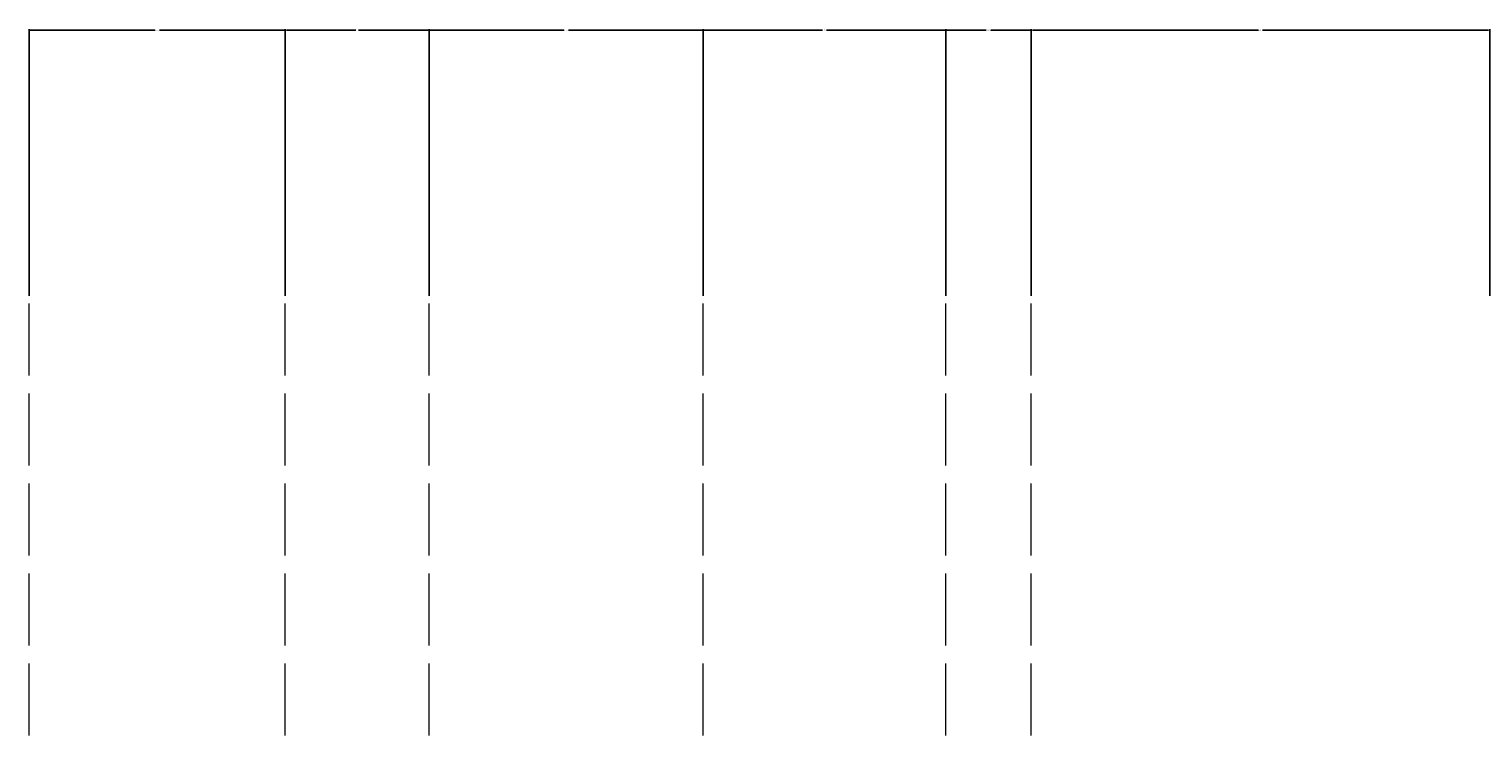
# Model space of a CAD drawing. Units: inches. Extents: x 1159 to 4240, y 1112 to 2085.
# Tile 7 of 13: x 1293 to 1535, y 1968 to 2085. Entities that reach past the tile are written whole.
import ezdxf

# ---------------------------------------------------------------- set-up
doc = ezdxf.new("R2010")
doc.units = ezdxf.units.IN
doc.linetypes.add('ACAD_ISO02W100', pattern=[15, 12, -3])
doc.layers.add('A-ANNO-DIMS', color=2, linetype='Continuous', lineweight=18)
doc.layers.add('A-GRID', color=8, linetype='ACAD_ISO02W100', lineweight=13)
doc.styles.get("Standard").update_dxf_attribs({"font": 'arial.ttf'})
doc.dimstyles.get("Standard").update_dxf_attribs({"dimtxt": 0.18, "dimasz": 0.18, "dimexe": 0.18, "dimexo": 0.0625, "dimgap": 0.09, "dimtad": 0, "dimtih": 1, "dimtoh": 1, "dimdec": 4, "dimzin": 0, "dimdsep": 46, "dimtxsty": 'Standard', "dimcen": 0.09, "dimadec": 0, "dimazin": 0, "dimtfac": 1, "dimtdec": 4, "dimtofl": 0, "dimtmove": 0, "dimatfit": 3, "dimfxl": 1, "dimtolj": 1, "dimtzin": 0, "dimarcsym": 0})

# ---------------------------------------------------------------- blocks, each defined once
blk = doc.blocks.new('HOUSE-35x60-SETTING-OUT-GRID')
for p, q in [((89.32, 0), (89.32, 883.25)), ((132.07, 0), (132.07, 883.25)), ((156.07, 0), (156.07, 883.25)), ((201.82, 0), (201.82, 883.25)), ((242.32, 0), (242.32, 883.25)), ((256.57, 0), (256.57, 883.25))]:
    blk.add_line(p, q)
blk = doc.blocks.new('*D26')
at = {"layer": 'A-ANNO-DIMS', "color": 0, "lineweight": -2, "transparency": 16777216}
for p, q in [((1292.63, 2040.27), (1292.63, 2084.73)), ((1292.81, 2084.55), (1313.6, 2084.55)), ((1335.2, 2084.55), (1314.4, 2084.55)), ((1335.38, 2040.27), (1335.38, 2084.73))]:
    blk.add_line(p, q, dxfattribs=at)
at = {"layer": 'A-ANNO-DIMS', "color": 0, "lineweight": 100, "transparency": 16777216}
for points in [[(1292.81, 2084.58), (1292.81, 2084.52), (1292.63, 2084.55)], [(1335.2, 2084.58), (1335.2, 2084.52), (1335.38, 2084.55)]]:
    blk.add_solid(points, dxfattribs=at)
at = {"layer": 'Defpoints', "color": 0, "lineweight": 100, "transparency": 16777216}
for p in [(1335.38, 2084.55), (1292.63, 2040.2), (1335.38, 2040.2)]:
    blk.add_point(p, dxfattribs=at)
at = {"layer": 'A-ANNO-DIMS', "color": 0, "transparency": 16777216, "insert": (1314, 2084.55), "char_height": 0.18, "attachment_point": 5}
blk.add_mtext('\\A1;42.75', dxfattribs=at)
blk = doc.blocks.new('*D27')
at = {"layer": 'A-ANNO-DIMS', "color": 0, "lineweight": -2, "transparency": 16777216}
for p, q in [((1335.38, 2040.27), (1335.38, 2084.73)), ((1335.56, 2084.55), (1347.16, 2084.55)), ((1359.2, 2084.55), (1347.6, 2084.55)), ((1359.38, 2040.27), (1359.38, 2084.73))]:
    blk.add_line(p, q, dxfattribs=at)
at = {"layer": 'A-ANNO-DIMS', "color": 0, "lineweight": 100, "transparency": 16777216}
for points in [[(1335.56, 2084.58), (1335.56, 2084.52), (1335.38, 2084.55)], [(1359.2, 2084.58), (1359.2, 2084.52), (1359.38, 2084.55)]]:
    blk.add_solid(points, dxfattribs=at)
at = {"layer": 'Defpoints', "color": 0, "lineweight": 100, "transparency": 16777216}
for p in [(1359.38, 2084.55), (1335.38, 2040.2), (1359.38, 2040.2)]:
    blk.add_point(p, dxfattribs=at)
at = {"layer": 'A-ANNO-DIMS', "color": 0, "transparency": 16777216, "insert": (1347.38, 2084.55), "char_height": 0.18, "attachment_point": 5}
blk.add_mtext('\\A1;24', dxfattribs=at)
blk = doc.blocks.new('*D28')
at = {"layer": 'A-ANNO-DIMS', "color": 0, "lineweight": -2, "transparency": 16777216}
for p, q in [((1359.38, 2040.27), (1359.38, 2084.73)), ((1359.56, 2084.55), (1381.85, 2084.55)), ((1404.95, 2084.55), (1382.65, 2084.55)), ((1405.13, 2040.27), (1405.13, 2084.73))]:
    blk.add_line(p, q, dxfattribs=at)
at = {"layer": 'A-ANNO-DIMS', "color": 0, "lineweight": 100, "transparency": 16777216}
for points in [[(1359.56, 2084.58), (1359.56, 2084.52), (1359.38, 2084.55)], [(1404.95, 2084.58), (1404.95, 2084.52), (1405.13, 2084.55)]]:
    blk.add_solid(points, dxfattribs=at)
at = {"layer": 'Defpoints', "color": 0, "lineweight": 100, "transparency": 16777216}
for p in [(1405.13, 2084.55), (1359.38, 2040.2), (1405.13, 2040.2)]:
    blk.add_point(p, dxfattribs=at)
at = {"layer": 'A-ANNO-DIMS', "color": 0, "transparency": 16777216, "insert": (1382.25, 2084.55), "char_height": 0.18, "attachment_point": 5}
blk.add_mtext('\\A1;45.75', dxfattribs=at)
blk = doc.blocks.new('*D29')
at = {"layer": 'A-ANNO-DIMS', "color": 0, "lineweight": -2, "transparency": 16777216}
for p, q in [((1405.13, 2040.27), (1405.13, 2084.73)), ((1405.31, 2084.55), (1425.05, 2084.55)), ((1445.45, 2084.55), (1425.7, 2084.55)), ((1445.63, 2040.27), (1445.63, 2084.73))]:
    blk.add_line(p, q, dxfattribs=at)
at = {"layer": 'A-ANNO-DIMS', "color": 0, "lineweight": 100, "transparency": 16777216}
for points in [[(1405.31, 2084.58), (1405.31, 2084.52), (1405.13, 2084.55)], [(1445.45, 2084.58), (1445.45, 2084.52), (1445.63, 2084.55)]]:
    blk.add_solid(points, dxfattribs=at)
at = {"layer": 'Defpoints', "color": 0, "lineweight": 100, "transparency": 16777216}
for p in [(1445.63, 2084.55), (1405.13, 2040.2), (1445.63, 2040.2)]:
    blk.add_point(p, dxfattribs=at)
at = {"layer": 'A-ANNO-DIMS', "color": 0, "transparency": 16777216, "insert": (1425.38, 2084.55), "char_height": 0.18, "attachment_point": 5}
blk.add_mtext('\\A1;40.5', dxfattribs=at)
blk = doc.blocks.new('*D30')
at = {"layer": 'A-ANNO-DIMS', "color": 0, "lineweight": -2, "transparency": 16777216}
for p, q in [((1445.63, 2040.27), (1445.63, 2084.73)), ((1445.81, 2084.55), (1452.36, 2084.55)), ((1459.7, 2084.55), (1453.14, 2084.55)), ((1459.88, 2040.27), (1459.88, 2084.73))]:
    blk.add_line(p, q, dxfattribs=at)
at = {"layer": 'A-ANNO-DIMS', "color": 0, "lineweight": 100, "transparency": 16777216}
for points in [[(1445.81, 2084.58), (1445.81, 2084.52), (1445.63, 2084.55)], [(1459.7, 2084.58), (1459.7, 2084.52), (1459.88, 2084.55)]]:
    blk.add_solid(points, dxfattribs=at)
at = {"layer": 'Defpoints', "color": 0, "lineweight": 100, "transparency": 16777216}
for p in [(1459.88, 2084.55), (1445.63, 2040.2), (1459.88, 2040.2)]:
    blk.add_point(p, dxfattribs=at)
at = {"layer": 'A-ANNO-DIMS', "color": 0, "transparency": 16777216, "insert": (1452.75, 2084.55), "char_height": 0.18, "attachment_point": 5}
blk.add_mtext('\\A1;14.25', dxfattribs=at)
blk = doc.blocks.new('*D31')
at = {"layer": 'A-ANNO-DIMS', "color": 0, "lineweight": -2, "transparency": 16777216}
for p, q in [((1459.88, 2040.27), (1459.88, 2084.73)), ((1460.06, 2084.55), (1497.8, 2084.55)), ((1536.2, 2084.55), (1498.45, 2084.55)), ((1536.38, 2040.27), (1536.38, 2084.73))]:
    blk.add_line(p, q, dxfattribs=at)
at = {"layer": 'A-ANNO-DIMS', "color": 0, "lineweight": 100, "transparency": 16777216}
for points in [[(1460.06, 2084.58), (1460.06, 2084.52), (1459.88, 2084.55)], [(1536.2, 2084.58), (1536.2, 2084.52), (1536.38, 2084.55)]]:
    blk.add_solid(points, dxfattribs=at)
at = {"layer": 'Defpoints', "color": 0, "lineweight": 100, "transparency": 16777216}
for p in [(1536.38, 2084.55), (1459.88, 2040.2), (1536.38, 2040.2)]:
    blk.add_point(p, dxfattribs=at)
at = {"layer": 'A-ANNO-DIMS', "color": 0, "transparency": 16777216, "insert": (1498.13, 2084.55), "char_height": 0.18, "attachment_point": 5}
blk.add_mtext('\\A1;76.5', dxfattribs=at)

msp = doc.modelspace()

# ---------------------------------------------------------------- block references
at = {"layer": 'A-GRID'}
msp.add_blockref('HOUSE-35x60-SETTING-OUT-GRID', (1203.31, 1156.954), dxfattribs=at)

# ---------------------------------------------------------------- dimensions: what is measured, and where the dimension line sits
at = {"layer": 'A-ANNO-DIMS'}
for base, p1, p2, override, picture, middle in [((1335.375, 2084.554), (1292.625, 2040.204), (1335.375, 2040.204), {"dimdec": 2, "dimlfac": 1, "dimrnd": 0, "dimzin": 0, "dimdsep": 46, "dimlunit": 2}, '*D26', (1314, 2084.554)), ((1359.375, 2084.554), (1335.375, 2040.204), (1359.375, 2040.204), {"dimdec": 0, "dimlfac": 1, "dimrnd": 0, "dimzin": 0, "dimdsep": 46, "dimlunit": 2}, '*D27', (1347.375, 2084.554)), ((1405.125, 2084.554), (1359.375, 2040.204), (1405.125, 2040.204), {"dimdec": 2, "dimlfac": 1, "dimrnd": 0, "dimzin": 0, "dimdsep": 46, "dimlunit": 2}, '*D28', (1382.25, 2084.554)), ((1445.625, 2084.554), (1405.125, 2040.204), (1445.625, 2040.204), {"dimdec": 1, "dimlfac": 1, "dimrnd": 0, "dimzin": 0, "dimdsep": 46, "dimlunit": 2}, '*D29', (1425.375, 2084.554)), ((1459.875, 2084.554), (1445.625, 2040.204), (1459.875, 2040.204), {"dimdec": 2, "dimlfac": 1, "dimrnd": 0, "dimzin": 0, "dimdsep": 46, "dimlunit": 2}, '*D30', (1452.75, 2084.554)), ((1536.375, 2084.554), (1459.875, 2040.204), (1536.375, 2040.204), {"dimdec": 1, "dimlfac": 1, "dimrnd": 0, "dimzin": 0, "dimdsep": 46, "dimlunit": 2}, '*D31', (1498.125, 2084.554))]:
    dim = msp.add_linear_dim(base=base, p1=p1, p2=p2, dimstyle='Standard', override=override, dxfattribs=at)
    dim.commit()
    dim.dimension.update_dxf_attribs({"geometry": picture, "text_midpoint": middle})

doc.saveas('drawing.dxf')
